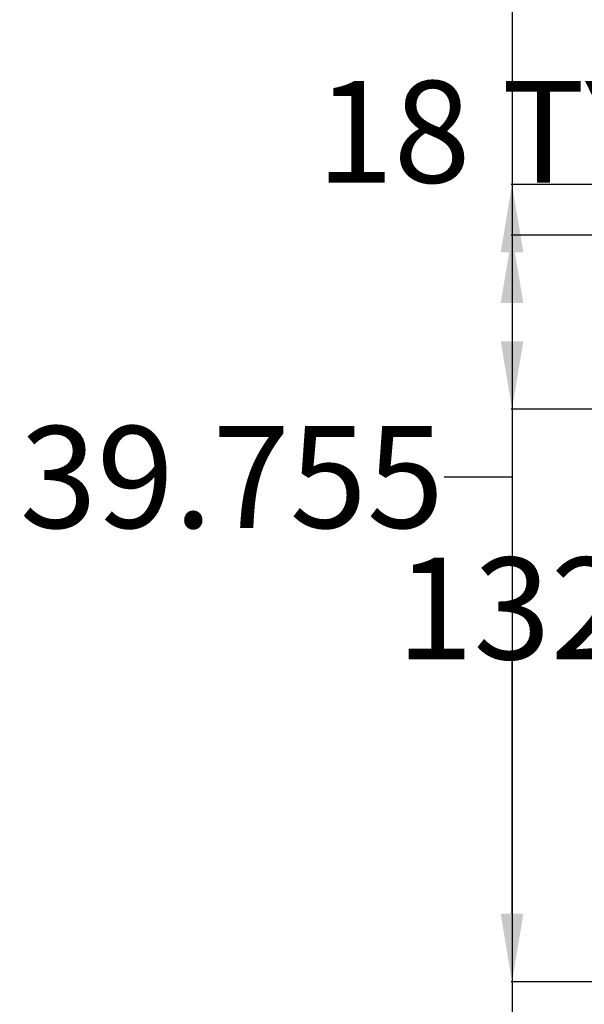
# Model space of a CAD drawing. Units: inches. Extents: x -90 to 536, y -553 to 299.
# Tile 16 of 27: x -90 to 10, y -2 to 173. Entities that reach past the tile are written whole.
import ezdxf

# ---------------------------------------------------------------- set-up
doc = ezdxf.new("R2010")
doc.units = ezdxf.units.IN
doc.layers.add('A-ANNO-DIMS', color=2, linetype='Continuous', lineweight=18)
doc.styles.get("Standard").update_dxf_attribs({"font": 'arial.ttf'})
doc.dimstyles.get("Standard").update_dxf_attribs({"dimtxt": 18, "dimasz": 12, "dimexe": 0.18, "dimexo": 0.0625, "dimgap": 0.09, "dimtad": 0, "dimtih": 1, "dimtoh": 1, "dimdec": 0, "dimzin": 0, "dimdsep": 46, "dimlunit": 3, "dimtxsty": 'Standard', "dimcen": 0.09, "dimadec": 0, "dimazin": 0, "dimtfac": 1, "dimtdec": 0, "dimtofl": 0, "dimtmove": 0, "dimatfit": 3, "dimfxl": 1, "dimtolj": 1, "dimtzin": 0, "dimarcsym": 0})

# ---------------------------------------------------------------- blocks, each defined once
blk = doc.blocks.new('*D32')
at = {"layer": 'A-ANNO-DIMS', "color": 0, "lineweight": -2, "transparency": 16777216}
for p, q in [((59.26, 152.75), (47.26, 152.75)), ((65.58, 142.54), (59.26, 152.75)), ((69.35, 130.76), (72.05, 132.44)), ((78.69, 115.67), (81.39, 117.34)), ((87.55, 107.05), (93.87, 96.84))]:
    blk.add_line(p, q, dxfattribs=at)
at = {"layer": 'A-ANNO-DIMS', "color": 0, "transparency": 16777216}
for points in [[(67.28, 143.6), (63.88, 141.49), (71.89, 132.34)], [(89.25, 108.1), (85.85, 105.99), (81.24, 117.25)]]:
    blk.add_solid(points, dxfattribs=at)
at = {"layer": 'Defpoints', "color": 0, "transparency": 16777216}
for p in [(71.89, 132.34), (69.29, 130.73), (78.63, 115.64)]:
    blk.add_point(p, dxfattribs=at)
at = {"layer": 'A-ANNO-DIMS', "color": 0, "transparency": 16777216, "insert": (4.21, 152.75), "char_height": 18, "attachment_point": 5}
blk.add_mtext('\\A1;18 TYP.', dxfattribs=at)
blk = doc.blocks.new('*D54')
at = {"layer": 'A-ANNO-DIMS', "color": 0, "lineweight": -2, "transparency": 16777216}
for p, q in [((113.07, 249.45), (-2.85, 249.45)), ((-2.67, 237.45), (-2.67, -117.77)), ((-2.67, -491.55), (-2.67, -136.34)), ((38.07, -503.55), (-2.85, -503.55))]:
    blk.add_line(p, q, dxfattribs=at)
at = {"layer": 'A-ANNO-DIMS', "color": 0, "transparency": 16777216}
for points in [[(-4.67, 237.45), (-0.67, 237.45), (-2.67, 249.45)], [(-4.67, -491.55), (-0.67, -491.55), (-2.67, -503.55)]]:
    blk.add_solid(points, dxfattribs=at)
at = {"layer": 'Defpoints', "color": 0, "transparency": 16777216}
for p in [(-2.67, 249.45), (113.13, 249.45), (38.13, -503.55)]:
    blk.add_point(p, dxfattribs=at)
at = {"layer": 'A-ANNO-DIMS', "color": 0, "transparency": 16777216, "insert": (-2.67, -127.05), "char_height": 18, "attachment_point": 5}
blk.add_mtext('\\A1;753', dxfattribs=at)
blk = doc.blocks.new('*D56')
at = {"layer": 'A-ANNO-DIMS', "color": 0, "lineweight": -2, "transparency": 16777216}
for p, q in [((47.07, 134.45), (-2.85, 134.45)), ((-2.67, 122.45), (-2.67, 77.73)), ((-2.67, 14.45), (-2.67, 59.16)), ((47.07, 2.45), (-2.85, 2.45))]:
    blk.add_line(p, q, dxfattribs=at)
at = {"layer": 'A-ANNO-DIMS', "color": 0, "transparency": 16777216}
for points in [[(-4.67, 122.45), (-0.67, 122.45), (-2.67, 134.45)], [(-4.67, 14.45), (-0.67, 14.45), (-2.67, 2.45)]]:
    blk.add_solid(points, dxfattribs=at)
at = {"layer": 'Defpoints', "color": 0, "transparency": 16777216}
for p in [(-2.67, 134.45), (47.13, 134.45), (47.13, 2.45)]:
    blk.add_point(p, dxfattribs=at)
at = {"layer": 'A-ANNO-DIMS', "color": 0, "transparency": 16777216, "insert": (-2.67, 68.45), "char_height": 18, "attachment_point": 5}
blk.add_mtext('\\A1;132', dxfattribs=at)
blk = doc.blocks.new('*D64')
at = {"layer": 'A-ANNO-DIMS', "color": 0, "lineweight": -2, "transparency": 16777216}
for p, q in [((38.07, 143.45), (-2.85, 143.45)), ((-2.67, 131.45), (-2.67, 115.69)), ((38.07, 103.69), (-2.85, 103.69)), ((-2.67, 103.69), (-2.67, 91.69)), ((-2.67, 91.69), (-14.67, 91.69))]:
    blk.add_line(p, q, dxfattribs=at)
at = {"layer": 'A-ANNO-DIMS', "color": 0, "transparency": 16777216}
for points in [[(-4.67, 131.45), (-0.67, 131.45), (-2.67, 143.45)], [(-4.67, 115.69), (-0.67, 115.69), (-2.67, 103.69)]]:
    blk.add_solid(points, dxfattribs=at)
at = {"layer": 'Defpoints', "color": 0, "transparency": 16777216}
for p in [(38.13, 143.45), (-2.67, 103.69), (38.13, 103.69)]:
    blk.add_point(p, dxfattribs=at)
at = {"layer": 'A-ANNO-DIMS', "color": 0, "transparency": 16777216, "insert": (-52.18, 91.69), "char_height": 18, "attachment_point": 5}
blk.add_mtext('\\A1;39.755', dxfattribs=at)

msp = doc.modelspace()

# ---------------------------------------------------------------- dimensions: what is measured, and where the dimension line sits
at = {"layer": 'A-ANNO-DIMS'}
for base, p1, p2, override, picture, middle in [((-2.6677, 249.4462), (38.1317, -503.5538), (113.1317, 249.4462), {"dimdec": 0, "dimlfac": 1, "dimrnd": 0, "dimzin": 0, "dimdsep": 46, "dimlunit": 2}, '*D54', (-2.6677, -127.0538)), ((-2.6677, 103.6916), (38.1317, 143.4462), (38.1317, 103.6916), {"dimdec": 3, "dimlfac": 1, "dimrnd": 0, "dimzin": 0, "dimdsep": 46, "dimlunit": 2}, '*D64', (-52.182, 91.6916)), ((-2.6677, 134.4462), (47.1317, 2.4462), (47.1317, 134.4462), {"dimdec": 0, "dimlfac": 1, "dimrnd": 0, "dimzin": 0, "dimdsep": 46, "dimlunit": 2}, '*D56', (-2.6677, 68.4462))]:
    dim = msp.add_linear_dim(base=base, p1=p1, p2=p2, angle=90, dimstyle='Standard', override=override, dxfattribs=at)
    dim.commit()
    dim.dimension.update_dxf_attribs({"geometry": picture, "text_midpoint": middle})
dim = msp.add_linear_dim(base=(71.8939, 132.3414), p1=(78.6344, 115.6404), p2=(69.2932, 130.7316), angle=121.756702, text='<> TYP.', dimstyle='Standard', override={"dimdec": 0, "dimlfac": 1, "dimrnd": 0, "dimzin": 0, "dimdsep": 46, "dimlunit": 2}, dxfattribs=at)
dim.commit()
dim.dimension.update_dxf_attribs({"geometry": '*D32', "text_midpoint": (4.2106, 152.7484)})

doc.saveas('drawing.dxf')
